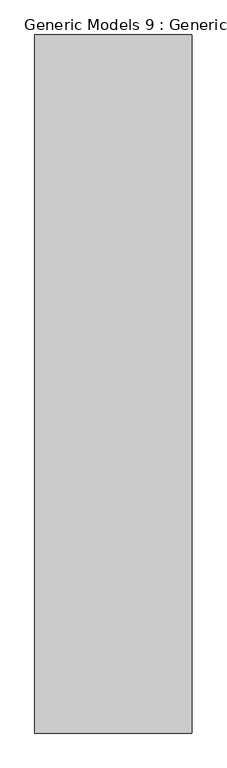
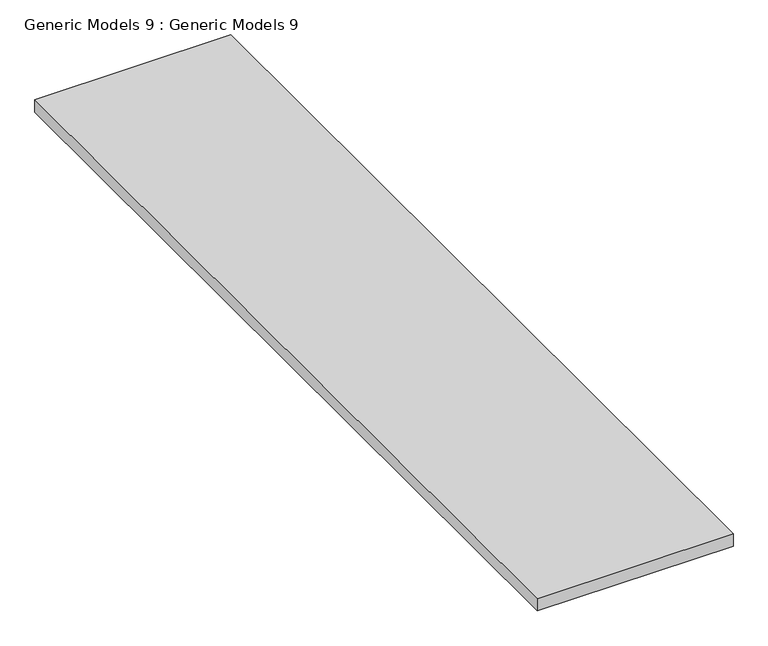
"""IFC4 building model written with IfcOpenShell, lengths in millimetres: proxy geometry, Generic Models 9 : Generic Models 9."""

from ifc_helpers import new_model, si_unit, frame, origin, place, context, project, spatial, polyline, outline, extrude, source, transform, mapped, element, save


def generic_models_9_generic_models_9_2e7d35d1(model_context):
    return source(origin(), model_context, "Body", "SweptSolid", [
        extrude(outline(polyline([(2800.2596873, -19148.6131479), (2800.2596873, -8904.6038063), (5108.5369073, -8904.6038063), (5108.5369073, -19148.6131479), (2800.2596873, -19148.6131479)])), frame((0.0, 0.0, -152.4), z_axis=(0.0, 0.0, 1.0), x_axis=(1.0, 0.0, 0.0)), (0.0, 0.0, 1.0), 152.4),
    ])


if __name__ == "__main__":
    model = new_model("IFC4")
    model_context = context("Model", 3, world=origin())
    ifc_project = project(units=[si_unit("LENGTHUNIT", "METRE", prefix="MILLI")], contexts=[model_context])
    site = spatial("IfcSite", under=ifc_project)
    building = spatial("IfcBuilding", under=site)
    placement = place(None, origin())
    generic_models_9_generic_models_9_shape = generic_models_9_generic_models_9_2e7d35d1(model_context)
    element("IfcBuildingElementProxy", 1, Name="Generic Models 9 : Generic Models 9", ObjectType="Generic Models 9 : Generic Models 9", at=placement, inside=building, context=model_context, shape_type="MappedRepresentation", body=[
        mapped(generic_models_9_generic_models_9_shape, transform((0.0, 0.0, 0.0), x_axis=(1.0, 0.0, 0.0), y_axis=(0.0, 1.0, 0.0), z_axis=(0.0, 0.0, 1.0))),
    ])
    save(model, "model.ifc")
